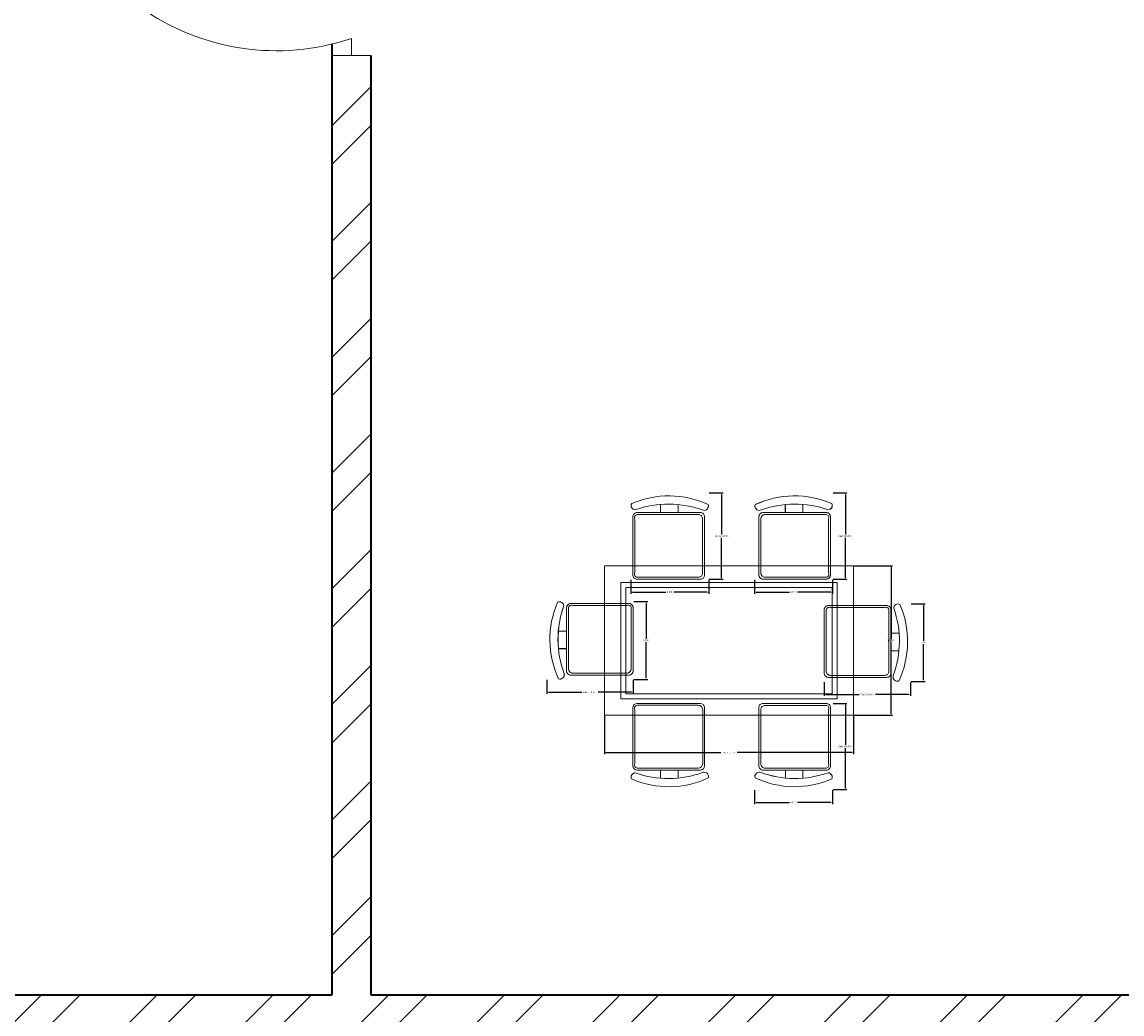
# Model space of a CAD drawing. Units: inches. Extents: x 2120 to 4013, y 1390 to 3019.
# Tile 31 of 59: x 2356 to 2484, y 2073 to 2188. Entities that reach past the tile are written whole.
import ezdxf

# ---------------------------------------------------------------- set-up
doc = ezdxf.new("R2010")
doc.units = ezdxf.units.IN
for name, color, linetype, lineweight in [('A-ANNO-DIMS', 2, 'Continuous', 18), ('A-DOOR', 3, 'Continuous', 18), ('A-FURN', 8, 'Continuous', 13), ('A-WALL', 7, 'Continuous', 35), ('A-WALL-PATT', 252, 'Continuous', 13)]:
    doc.layers.add(name, color=color, linetype=linetype, lineweight=lineweight)
doc.styles.get("Standard").update_dxf_attribs({"font": 'arial.ttf'})
doc.dimstyles.get("Standard").update_dxf_attribs({"dimtxt": 0.18, "dimasz": 0.18, "dimexe": 0.18, "dimexo": 0.0625, "dimgap": 0.09, "dimtad": 0, "dimtih": 1, "dimtoh": 1, "dimdec": 4, "dimzin": 0, "dimdsep": 46, "dimtxsty": 'Standard', "dimcen": 0.09, "dimadec": 0, "dimazin": 0, "dimtfac": 1, "dimtdec": 4, "dimtofl": 0, "dimtmove": 0, "dimatfit": 3, "dimfxl": 1, "dimtolj": 1, "dimtzin": 0, "dimarcsym": 0})

# ---------------------------------------------------------------- blocks, each defined once
blk = doc.blocks.new('DOOR-SWING-36IN-108p68DEG')
for p, q in [((38.25, 29.83), (33.75, 29.83)), ((33.75, 29.83), (36, 29.83)), ((36, 29.83), (36, 27.83)), ((36, 27.83), (0, 27.83)), ((36, 0), (36, 2)), ((33.75, 0), (38.25, 0)), ((38.25, 0), (36, 0))]:
    blk.add_line(p, q)
blk.add_arc((27.27, 27.83), 27.27, 180, 288.6764)
blk = doc.blocks.new('TABLE-DINING')
for points in [[(0, 17.41), (29.01, 17.41), (29.01, 0), (0, 0)], [(1.93, 15.47), (27.08, 15.47), (27.08, 1.93), (1.93, 1.93)], [(2.51, 14.89), (26.5, 14.89), (26.5, 2.51), (2.51, 2.51)]]:
    blk.add_lwpolyline(points, close=True)
blk = doc.blocks.new('CHAIR-DINING-01')
for points in [[(1.68, 0.62, -0.578392), (1.02, 0.02, -0.214524), (0.9, 8.94, -0.552014), (1.62, 8.52, 0.175809), (1.68, 0.62)], [(1.93, 8.29, -0.414214), (2.45, 8.81), (9.19, 8.81, -0.414214), (9.7, 8.29), (9.7, 0.96, -0.414214), (9.19, 0.45), (2.45, 0.45, -0.414214), (1.93, 0.96), (1.93, 8.29)], [(1.93, 3.54), (1.01, 3.54, 0.064759)]]:
    blk.add_lwpolyline(points, format="xyb")
blk.add_lwpolyline([(2.16, 8.29), (2.16, 1.19, 0.414214), (2.68, 0.68), (8.96, 0.68, 0.414214), (9.47, 1.19), (9.47, 8.29, 0.512069), (8.96, 8.58), (2.68, 8.58, 0.512069)], format="xyb", close=True)
blk.add_lwpolyline([(0.99, 5.59), (1.93, 5.59)])
blk = doc.blocks.new('CHAIR-DINING-02')
for points in [[(8.09, 8.52, -0.175809), (8.03, 0.62, 0.578392), (8.69, 0.02, 0.214524), (8.81, 8.94, 0.552014), (8.09, 8.52, -0.065079)], [(7.77, 8.29, 0.414214), (7.26, 8.81), (0.51, 8.81, 0.414214), (0, 8.29), (0, 0.96, 0.414214), (0.51, 0.45), (7.26, 0.45, 0.414214), (7.77, 0.96), (7.77, 8.29)], [(7.77, 3.54), (8.7, 3.54, -0.064759)]]:
    blk.add_lwpolyline(points, format="xyb")
blk.add_lwpolyline([(7.54, 8.29), (7.54, 1.19, -0.414214), (7.03, 0.68), (0.74, 0.68, -0.414214), (0.23, 1.19), (0.23, 8.29, -0.512069), (0.74, 8.58), (7.03, 8.58, -0.512069)], format="xyb", close=True)
blk.add_lwpolyline([(8.72, 5.59), (7.77, 5.59)])
blk = doc.blocks.new('CHAIR-DINING-03')
for points in [[(8.29, 1.93, 0.414214), (8.81, 2.45), (8.81, 9.19, 0.414214), (8.29, 9.7), (0.96, 9.7, 0.414214), (0.45, 9.19), (0.45, 2.45, 0.414214), (0.96, 1.93), (8.29, 1.93)], [(8.52, 1.62, -0.175809), (0.62, 1.68, 0.578392), (0.02, 1.02, 0.214524), (8.94, 0.9, 0.552014), (8.52, 1.62, -0.065079)], [(3.54, 1.93), (3.54, 1.01, -0.064759)]]:
    blk.add_lwpolyline(points, format="xyb")
blk.add_lwpolyline([(8.29, 2.16), (1.19, 2.16, -0.414214), (0.68, 2.68), (0.68, 8.96, -0.414214), (1.19, 9.47), (8.29, 9.47, -0.512069), (8.58, 8.96), (8.58, 2.68, -0.512069)], format="xyb", close=True)
blk.add_lwpolyline([(5.59, 0.99), (5.59, 1.93)])
blk = doc.blocks.new('CHAIR-DINING-09')
for points in [[(0.47, 8.09, -0.175809), (8.38, 8.03, 0.578392), (8.97, 8.69, 0.214524), (0.06, 8.81, 0.552014), (0.47, 8.09, -0.065079)], [(8.04, 7.77), (0.71, 7.77, 0.414214), (0.19, 7.26), (0.19, 0.51, 0.414214), (0.71, 0), (8.04, 0, 0.414214), (8.55, 0.51), (8.55, 7.26, 0.414214), (8.04, 7.77)], [(5.46, 7.77), (5.46, 8.7, -0.064759)]]:
    blk.add_lwpolyline(points, format="xyb")
blk.add_lwpolyline([(3.41, 8.72), (3.41, 7.77)])
blk.add_lwpolyline([(0.71, 7.54), (7.81, 7.54, -0.414214), (8.32, 7.03), (8.32, 0.74, -0.414214), (7.81, 0.23), (0.71, 0.23, -0.512069), (0.42, 0.74), (0.42, 7.03, -0.512069)], format="xyb", close=True)
blk = doc.blocks.new('CHAIR-DINING-10')
for points in [[(0.62, 8.03, -0.578392), (0.02, 8.69, -0.214524), (8.94, 8.81, -0.552014), (8.52, 8.09, 0.175809), (0.62, 8.03)], [(8.29, 7.77, -0.414214), (8.81, 7.26), (8.81, 0.51, -0.414214), (8.29, 0), (0.96, 0, -0.414214), (0.45, 0.51), (0.45, 7.26, -0.414214), (0.96, 7.77), (8.29, 7.77)], [(3.54, 7.77), (3.54, 8.7, 0.064759)]]:
    blk.add_lwpolyline(points, format="xyb")
blk.add_lwpolyline([(5.59, 8.72), (5.59, 7.77)])
blk.add_lwpolyline([(8.29, 7.54), (1.19, 7.54, 0.414214), (0.68, 7.03), (0.68, 0.74, 0.414214), (1.19, 0.23), (8.29, 0.23, 0.512069), (8.58, 0.74), (8.58, 7.03, 0.512069)], format="xyb", close=True)
blk = doc.blocks.new('CHAIR-DINING-11')
for points in [[(0.47, 8.09, -0.175809), (8.38, 8.03, 0.578392), (8.97, 8.69, 0.214524), (0.06, 8.81, 0.552014), (0.47, 8.09, -0.065079)], [(8.04, 7.77), (0.71, 7.77, 0.414214), (0.19, 7.26), (0.19, 0.51, 0.414214), (0.71, 0), (8.04, 0, 0.414214), (8.55, 0.51), (8.55, 7.26, 0.414214), (8.04, 7.77)], [(5.46, 7.77), (5.46, 8.7, -0.064759)]]:
    blk.add_lwpolyline(points, format="xyb")
blk.add_lwpolyline([(3.41, 8.72), (3.41, 7.77)])
blk.add_lwpolyline([(0.71, 7.54), (7.81, 7.54, -0.414214), (8.32, 7.03), (8.32, 0.74, -0.414214), (7.81, 0.23), (0.71, 0.23, -0.512069), (0.42, 0.74), (0.42, 7.03, -0.512069)], format="xyb", close=True)
blk = doc.blocks.new('CHAIR-DINING-12')
for points in [[(8.09, 8.52, -0.175809), (8.03, 0.62, 0.578392), (8.69, 0.02, 0.214524), (8.81, 8.94, 0.552014), (8.09, 8.52, -0.065079)], [(7.77, 8.29, 0.414214), (7.26, 8.81), (0.51, 8.81, 0.414214), (0, 8.29), (0, 0.96, 0.414214), (0.51, 0.45), (7.26, 0.45, 0.414214), (7.77, 0.96), (7.77, 8.29)], [(7.77, 3.54), (8.7, 3.54, -0.064759)]]:
    blk.add_lwpolyline(points, format="xyb")
blk.add_lwpolyline([(7.54, 8.29), (7.54, 1.19, -0.414214), (7.03, 0.68), (0.74, 0.68, -0.414214), (0.23, 1.19), (0.23, 8.29, -0.512069), (0.74, 8.58), (7.03, 8.58, -0.512069)], format="xyb", close=True)
blk.add_lwpolyline([(8.72, 5.59), (7.77, 5.59)])
blk = doc.blocks.new('*D75')
at = {"layer": 'A-ANNO-DIMS', "color": 0, "lineweight": -2, "transparency": 16777216}
for p, q in [((2423.42, 2107.5), (2423.42, 2103.03)), ((2452.43, 2107.5), (2452.43, 2103.03)), ((2423.6, 2103.21), (2436.97, 2103.21)), ((2452.25, 2103.21), (2438.89, 2103.21))]:
    blk.add_line(p, q, dxfattribs=at)
at = {"layer": 'A-ANNO-DIMS', "color": 0, "transparency": 16777216}
for points in [[(2423.6, 2103.24), (2423.6, 2103.18), (2423.42, 2103.21)], [(2452.25, 2103.24), (2452.25, 2103.18), (2452.43, 2103.21)]]:
    blk.add_solid(points, dxfattribs=at)
at = {"layer": 'Defpoints', "color": 0, "transparency": 16777216}
for p in [(2423.42, 2107.56), (2452.43, 2107.56), (2452.43, 2103.21)]:
    blk.add_point(p, dxfattribs=at)
at = {"layer": 'A-ANNO-DIMS', "color": 0, "transparency": 16777216, "insert": (2437.93, 2103.21), "char_height": 0.18, "attachment_point": 5}
blk.add_mtext('\\A1;TABLE 29 TYP.', dxfattribs=at)
blk = doc.blocks.new('*D76')
at = {"layer": 'A-ANNO-DIMS', "color": 0, "lineweight": -2, "transparency": 16777216}
for p, q in [((2452.5, 2124.97), (2456.97, 2124.97)), ((2456.79, 2124.79), (2456.79, 2116.45)), ((2456.79, 2107.74), (2456.79, 2116.09)), ((2452.5, 2107.56), (2456.97, 2107.56))]:
    blk.add_line(p, q, dxfattribs=at)
at = {"layer": 'A-ANNO-DIMS', "color": 0, "transparency": 16777216}
for points in [[(2456.76, 2124.79), (2456.82, 2124.79), (2456.79, 2124.97)], [(2456.76, 2107.74), (2456.82, 2107.74), (2456.79, 2107.56)]]:
    blk.add_solid(points, dxfattribs=at)
at = {"layer": 'Defpoints', "color": 0, "transparency": 16777216}
for p in [(2452.43, 2124.97), (2456.79, 2124.97), (2452.43, 2107.56)]:
    blk.add_point(p, dxfattribs=at)
at = {"layer": 'A-ANNO-DIMS', "color": 0, "transparency": 16777216, "insert": (2456.79, 2116.27), "char_height": 0.18, "attachment_point": 5}
blk.add_mtext('\\A1;17 TYP.', dxfattribs=at)
blk = doc.blocks.new('*D81')
at = {"layer": 'A-ANNO-DIMS', "color": 0, "lineweight": -2, "transparency": 16777216}
for p, q in [((2416.73, 2111.68), (2416.73, 2110.06)), ((2426.77, 2111.68), (2426.77, 2110.06)), ((2416.91, 2110.24), (2420.8, 2110.24)), ((2426.59, 2110.24), (2422.7, 2110.24))]:
    blk.add_line(p, q, dxfattribs=at)
at = {"layer": 'A-ANNO-DIMS', "color": 0, "transparency": 16777216}
for points in [[(2416.91, 2110.27), (2416.91, 2110.21), (2416.73, 2110.24)], [(2426.59, 2110.27), (2426.59, 2110.21), (2426.77, 2110.24)]]:
    blk.add_solid(points, dxfattribs=at)
at = {"layer": 'Defpoints', "color": 0, "transparency": 16777216}
for p in [(2416.73, 2111.74), (2426.77, 2111.74), (2426.77, 2110.24)]:
    blk.add_point(p, dxfattribs=at)
at = {"layer": 'A-ANNO-DIMS', "color": 0, "transparency": 16777216, "insert": (2421.75, 2110.24), "char_height": 0.18, "attachment_point": 5}
blk.add_mtext('\\A1;CHAIR 10 TYP.', dxfattribs=at)
blk = doc.blocks.new('*D82')
at = {"layer": 'A-ANNO-DIMS', "color": 0, "lineweight": -2, "transparency": 16777216}
for p, q in [((2426.84, 2120.8), (2428.46, 2120.8)), ((2428.28, 2120.62), (2428.28, 2116.45)), ((2428.28, 2111.92), (2428.28, 2116.09)), ((2426.84, 2111.74), (2428.46, 2111.74))]:
    blk.add_line(p, q, dxfattribs=at)
at = {"layer": 'A-ANNO-DIMS', "color": 0, "transparency": 16777216}
for points in [[(2428.25, 2120.62), (2428.31, 2120.62), (2428.28, 2120.8)], [(2428.25, 2111.92), (2428.31, 2111.92), (2428.28, 2111.74)]]:
    blk.add_solid(points, dxfattribs=at)
at = {"layer": 'Defpoints', "color": 0, "transparency": 16777216}
for p in [(2426.77, 2120.8), (2428.28, 2120.8), (2426.77, 2111.74)]:
    blk.add_point(p, dxfattribs=at)
at = {"layer": 'A-ANNO-DIMS', "color": 0, "transparency": 16777216, "insert": (2428.28, 2116.27), "char_height": 0.18, "attachment_point": 5}
blk.add_mtext('\\A1;9 TYP.', dxfattribs=at)
blk = doc.blocks.new('*D85')
at = {"layer": 'A-ANNO-DIMS', "color": 0, "lineweight": -2, "transparency": 16777216}
for p, q in [((2450.03, 2108.95), (2451.65, 2108.95)), ((2451.47, 2108.77), (2451.47, 2104.11)), ((2451.47, 2099.09), (2451.47, 2103.75)), ((2450.03, 2098.91), (2451.65, 2098.91))]:
    blk.add_line(p, q, dxfattribs=at)
at = {"layer": 'A-ANNO-DIMS', "color": 0, "transparency": 16777216}
for points in [[(2451.44, 2108.77), (2451.5, 2108.77), (2451.47, 2108.95)], [(2451.44, 2099.09), (2451.5, 2099.09), (2451.47, 2098.91)]]:
    blk.add_solid(points, dxfattribs=at)
at = {"layer": 'Defpoints', "color": 0, "transparency": 16777216}
for p in [(2449.96, 2108.95), (2451.47, 2108.95), (2449.96, 2098.91)]:
    blk.add_point(p, dxfattribs=at)
at = {"layer": 'A-ANNO-DIMS', "color": 0, "transparency": 16777216, "insert": (2451.47, 2103.93), "char_height": 0.18, "attachment_point": 5}
blk.add_mtext('\\A1;CHAIR 10 TYP.', dxfattribs=at)
blk = doc.blocks.new('*D86')
at = {"layer": 'A-ANNO-DIMS', "color": 0, "lineweight": -2, "transparency": 16777216}
for p, q in [((2440.91, 2098.85), (2440.91, 2097.22)), ((2449.96, 2098.85), (2449.96, 2097.22)), ((2441.09, 2097.4), (2444.98, 2097.4)), ((2449.78, 2097.4), (2445.9, 2097.4))]:
    blk.add_line(p, q, dxfattribs=at)
at = {"layer": 'A-ANNO-DIMS', "color": 0, "transparency": 16777216}
for points in [[(2441.09, 2097.43), (2441.09, 2097.37), (2440.91, 2097.4)], [(2449.78, 2097.43), (2449.78, 2097.37), (2449.96, 2097.4)]]:
    blk.add_solid(points, dxfattribs=at)
at = {"layer": 'Defpoints', "color": 0, "transparency": 16777216}
for p in [(2440.91, 2098.91), (2449.96, 2098.91), (2449.96, 2097.4)]:
    blk.add_point(p, dxfattribs=at)
at = {"layer": 'A-ANNO-DIMS', "color": 0, "transparency": 16777216, "insert": (2445.44, 2097.4), "char_height": 0.18, "attachment_point": 5}
blk.add_mtext('\\A1;9 TYP.', dxfattribs=at)
blk = doc.blocks.new('*D97')
at = {"layer": 'A-ANNO-DIMS', "color": 0, "lineweight": -2, "transparency": 16777216}
for p, q in [((2435.63, 2133.44), (2437.25, 2133.44)), ((2437.07, 2133.26), (2437.07, 2128.6)), ((2437.07, 2123.57), (2437.07, 2128.23)), ((2435.63, 2123.39), (2437.25, 2123.39))]:
    blk.add_line(p, q, dxfattribs=at)
at = {"layer": 'A-ANNO-DIMS', "color": 0, "transparency": 16777216}
for points in [[(2437.04, 2133.26), (2437.1, 2133.26), (2437.07, 2133.44)], [(2437.04, 2123.57), (2437.1, 2123.57), (2437.07, 2123.39)]]:
    blk.add_solid(points, dxfattribs=at)
at = {"layer": 'Defpoints', "color": 0, "transparency": 16777216}
for p in [(2435.57, 2133.44), (2437.07, 2133.44), (2435.57, 2123.39)]:
    blk.add_point(p, dxfattribs=at)
at = {"layer": 'A-ANNO-DIMS', "color": 0, "transparency": 16777216, "insert": (2437.07, 2128.41), "char_height": 0.18, "attachment_point": 5}
blk.add_mtext('\\A1;CHAIR 10 TYP.', dxfattribs=at)
blk = doc.blocks.new('*D98')
at = {"layer": 'A-ANNO-DIMS', "color": 0, "lineweight": -2, "transparency": 16777216}
for p, q in [((2426.51, 2123.33), (2426.51, 2121.71)), ((2435.57, 2123.33), (2435.57, 2121.71)), ((2426.69, 2121.89), (2430.58, 2121.89)), ((2435.39, 2121.89), (2431.5, 2121.89))]:
    blk.add_line(p, q, dxfattribs=at)
at = {"layer": 'A-ANNO-DIMS', "color": 0, "transparency": 16777216}
for points in [[(2426.69, 2121.92), (2426.69, 2121.86), (2426.51, 2121.89)], [(2435.39, 2121.92), (2435.39, 2121.86), (2435.57, 2121.89)]]:
    blk.add_solid(points, dxfattribs=at)
at = {"layer": 'Defpoints', "color": 0, "transparency": 16777216}
for p in [(2426.51, 2123.39), (2435.57, 2123.39), (2435.57, 2121.89)]:
    blk.add_point(p, dxfattribs=at)
at = {"layer": 'A-ANNO-DIMS', "color": 0, "transparency": 16777216, "insert": (2431.04, 2121.89), "char_height": 0.18, "attachment_point": 5}
blk.add_mtext('\\A1;9 TYP.', dxfattribs=at)
blk = doc.blocks.new('*D99')
at = {"layer": 'A-ANNO-DIMS', "color": 0, "lineweight": -2, "transparency": 16777216}
for p, q in [((2450.03, 2133.44), (2451.65, 2133.44)), ((2451.47, 2133.26), (2451.47, 2128.6)), ((2451.47, 2123.57), (2451.47, 2128.23)), ((2450.03, 2123.39), (2451.65, 2123.39))]:
    blk.add_line(p, q, dxfattribs=at)
at = {"layer": 'A-ANNO-DIMS', "color": 0, "transparency": 16777216}
for points in [[(2451.44, 2133.26), (2451.5, 2133.26), (2451.47, 2133.44)], [(2451.44, 2123.57), (2451.5, 2123.57), (2451.47, 2123.39)]]:
    blk.add_solid(points, dxfattribs=at)
at = {"layer": 'Defpoints', "color": 0, "transparency": 16777216}
for p in [(2449.96, 2133.44), (2451.47, 2133.44), (2449.96, 2123.39)]:
    blk.add_point(p, dxfattribs=at)
at = {"layer": 'A-ANNO-DIMS', "color": 0, "transparency": 16777216, "insert": (2451.47, 2128.41), "char_height": 0.18, "attachment_point": 5}
blk.add_mtext('\\A1;CHAIR 10 TYP.', dxfattribs=at)
blk = doc.blocks.new('*D100')
at = {"layer": 'A-ANNO-DIMS', "color": 0, "lineweight": -2, "transparency": 16777216}
for p, q in [((2440.91, 2123.33), (2440.91, 2121.71)), ((2449.96, 2123.33), (2449.96, 2121.71)), ((2441.09, 2121.89), (2444.98, 2121.89)), ((2449.78, 2121.89), (2445.9, 2121.89))]:
    blk.add_line(p, q, dxfattribs=at)
at = {"layer": 'A-ANNO-DIMS', "color": 0, "transparency": 16777216}
for points in [[(2441.09, 2121.92), (2441.09, 2121.86), (2440.91, 2121.89)], [(2449.78, 2121.92), (2449.78, 2121.86), (2449.96, 2121.89)]]:
    blk.add_solid(points, dxfattribs=at)
at = {"layer": 'Defpoints', "color": 0, "transparency": 16777216}
for p in [(2440.91, 2123.39), (2449.96, 2123.39), (2449.96, 2121.89)]:
    blk.add_point(p, dxfattribs=at)
at = {"layer": 'A-ANNO-DIMS', "color": 0, "transparency": 16777216, "insert": (2445.44, 2121.89), "char_height": 0.18, "attachment_point": 5}
blk.add_mtext('\\A1;9 TYP.', dxfattribs=at)
blk = doc.blocks.new('*D103')
at = {"layer": 'A-ANNO-DIMS', "color": 0, "lineweight": -2, "transparency": 16777216}
for p, q in [((2449.01, 2111.43), (2449.01, 2109.81)), ((2459.05, 2111.43), (2459.05, 2109.81)), ((2449.19, 2109.99), (2453.08, 2109.99)), ((2458.87, 2109.99), (2454.98, 2109.99))]:
    blk.add_line(p, q, dxfattribs=at)
at = {"layer": 'A-ANNO-DIMS', "color": 0, "transparency": 16777216}
for points in [[(2449.19, 2110.02), (2449.19, 2109.96), (2449.01, 2109.99)], [(2458.87, 2110.02), (2458.87, 2109.96), (2459.05, 2109.99)]]:
    blk.add_solid(points, dxfattribs=at)
at = {"layer": 'Defpoints', "color": 0, "transparency": 16777216}
for p in [(2449.01, 2111.49), (2459.05, 2111.49), (2459.05, 2109.99)]:
    blk.add_point(p, dxfattribs=at)
at = {"layer": 'A-ANNO-DIMS', "color": 0, "transparency": 16777216, "insert": (2454.03, 2109.99), "char_height": 0.18, "attachment_point": 5}
blk.add_mtext('\\A1;CHAIR 10 TYP.', dxfattribs=at)
blk = doc.blocks.new('*D104')
at = {"layer": 'A-ANNO-DIMS', "color": 0, "lineweight": -2, "transparency": 16777216}
for p, q in [((2459.11, 2120.55), (2460.74, 2120.55)), ((2460.56, 2120.37), (2460.56, 2116.2)), ((2460.56, 2111.67), (2460.56, 2115.84)), ((2459.11, 2111.49), (2460.74, 2111.49))]:
    blk.add_line(p, q, dxfattribs=at)
at = {"layer": 'A-ANNO-DIMS', "color": 0, "transparency": 16777216}
for points in [[(2460.53, 2120.37), (2460.59, 2120.37), (2460.56, 2120.55)], [(2460.53, 2111.67), (2460.59, 2111.67), (2460.56, 2111.49)]]:
    blk.add_solid(points, dxfattribs=at)
at = {"layer": 'Defpoints', "color": 0, "transparency": 16777216}
for p in [(2459.05, 2120.55), (2460.56, 2120.55), (2459.05, 2111.49)]:
    blk.add_point(p, dxfattribs=at)
at = {"layer": 'A-ANNO-DIMS', "color": 0, "transparency": 16777216, "insert": (2460.56, 2116.02), "char_height": 0.18, "attachment_point": 5}
blk.add_mtext('\\A1;9 TYP.', dxfattribs=at)

msp = doc.modelspace()

# ---------------------------------------------------------------- hatches: boundary and pattern name
at = {"layer": 'A-WALL-PATT'}
h = msp.add_hatch(dxfattribs=at)
h.set_pattern_fill('ANSI32', color=256)
h.paths.add_polyline_path([(2271.7331, 2122.6377), (2262.7331, 2122.6377), (2262.7331, 2040.3893), (2267.2331, 2040.3893), (2271.7331, 2040.3893), (2271.7331, 2044.8856), (2271.7331, 2070.531), (2391.7331, 2070.531), (2391.7331, 1926.5306), (2388.3993, 1926.5306), (2388.3993, 1922.531), (2395.7331, 1922.531), (2395.7331, 1992.531), (2400.4511, 1992.531), (2400.4511, 1997.0306), (2395.7331, 1997.0306), (2395.7331, 2070.531), (2443.7331, 2070.531), (2443.7331, 2046.1368), (2448.2331, 2046.1368), (2448.2331, 2070.531), (2580.2331, 2070.531), (2580.2331, 1997.0306), (2492.9076, 1997.0306), (2492.9076, 1992.531), (2580.2331, 1992.531), (2580.2331, 1983.9368), (2589.2331, 1983.9368), (2589.2331, 2070.531), (2589.2331, 2075.0306), (2396.2331, 2075.0306), (2396.2331, 2184.3565), (2393.9831, 2184.3565), (2391.7331, 2184.3565), (2391.7331, 2075.0306), (2271.7331, 2075.0306)])
h.paths.add_polyline_path([(2724.7331, 2138.0306), (2628.7331, 2138.0306), (2628.7331, 2070.5306), (2628.7331, 2067.0987), (2633.2331, 2067.0987), (2637.7331, 2067.0987), (2637.7331, 2070.531), (2657.3413, 2070.531), (2657.3413, 2079.5306), (2637.7331, 2079.5306), (2637.7331, 2129.031), (2715.7331, 2129.031), (2715.7331, 2079.5306), (2698.0378, 2079.5306), (2698.0378, 2070.531), (2715.7331, 2070.531), (2715.7331, 2012.1531), (2720.2331, 2012.1531), (2724.7331, 2012.1531)])
h.paths.add_polyline_path([(2724.7331, 2213.031), (2831.3209, 2213.031), (2831.3209, 2215.281), (2831.3209, 2217.5306), (2724.7331, 2217.5306), (2724.7331, 2343.531), (2751.8755, 2343.531), (2751.8755, 2352.5306), (2715.7331, 2352.5306), (2715.7331, 2138.031), (2724.7331, 2138.031)])
h.paths.add_polyline_path([(2902.53, 2352.5306), (2811.8755, 2352.5306), (2811.8755, 2343.531), (2867.2331, 2343.531), (2867.2331, 2217.5306), (2863.6364, 2217.5306), (2863.6364, 2213.031), (2871.7331, 2213.031), (2871.7331, 2217.531), (2871.7331, 2343.531), (2902.53, 2343.531)])
h.paths.add_polyline_path([(3009.7331, 2352.5306), (2938.53, 2352.5306), (2938.53, 2343.531), (2966.2331, 2343.531), (2966.2331, 2242.3281), (2968.4831, 2242.3281), (2970.7331, 2242.3281), (2970.7331, 2343.531), (3009.7331, 2343.531)])
h.paths.add_polyline_path([(3009.7331, 2217.5306), (2970.7331, 2217.5306), (2970.7331, 2220.5422), (2968.4831, 2220.5422), (2966.2331, 2220.5422), (2966.2331, 2217.5306), (2911.7752, 2217.5306), (2907.7331, 2217.5306), (2907.7331, 2213.0306), (2907.7331, 2194.9663), (2912.2331, 2194.9663), (2912.2331, 2213.031), (2970.7331, 2213.031), (3000.7331, 2213.031), (3000.7331, 2205.523), (3009.7331, 2205.523)])
h.paths.add_polyline_path([(3009.7331, 2181.5227), (3000.7331, 2181.5227), (3000.7331, 2165.0306), (2912.2331, 2165.0306), (2912.2331, 2170.8202), (2907.7331, 2170.8202), (2907.7331, 2165.0306), (2899.5169, 2165.0306), (2899.5169, 2162.7806), (2899.5169, 2160.531), (2907.7331, 2160.531), (2907.7331, 2137.3432), (2912.2331, 2137.3432), (2912.2331, 2160.531), (3000.7331, 2160.531), (3000.7331, 2150.4993), (3009.7331, 2150.4993)])
h.paths.add_polyline_path([(3009.7331, 2126.499), (3005.2331, 2126.499), (3000.7331, 2126.499), (3000.7331, 2112.5306), (2912.2331, 2112.5306), (2912.2331, 2115.6036), (2907.7331, 2115.6036), (2907.7331, 2108.031), (3000.7331, 2108.031), (3000.7331, 2084.7256), (3009.7331, 2084.7256)], flags=17)
h.paths.add_polyline_path([(3009.7331, 1971.531), (3009.7331, 2024.7253), (3000.7331, 2024.7253), (3000.7331, 2006.4153), (3000.7331, 1971.5306), (2864.2331, 1971.5306), (2864.2331, 2160.531), (2868.0522, 2160.531), (2868.0522, 2165.0306), (2859.7331, 2165.0306), (2859.7331, 1971.5306), (2724.7331, 1971.5306), (2724.7331, 1977.7012), (2715.7331, 1977.7012), (2715.7331, 1962.5306), (2715.7331, 1950.9035), (2720.2331, 1950.9035), (2724.7331, 1950.9035), (2724.7331, 1962.531), (2855.2331, 1962.531), (2859.7331, 1962.531), (2859.7331, 1835.031), (2864.2331, 1834.8158), (2864.2331, 1962.531), (2958.7331, 1962.531), (2958.7331, 1937.0925), (2963.2331, 1937.0925), (2963.2331, 1962.531), (3000.7331, 1962.531), (3009.7331, 1962.531)])
h.paths.add_polyline_path([(2724.7331, 1728.531), (2822.7164, 1728.531), (2822.7164, 1733.0306), (2724.7331, 1733.0306), (2724.7331, 1779.3416), (2715.7331, 1779.3416), (2715.7331, 1581.531), (2753.02, 1581.531), (2753.02, 1586.031), (2753.02, 1590.5306), (2724.7331, 1590.5306)])
h.paths.add_polyline_path([(2864.2331, 1590.531), (2864.2331, 1787.031), (2868.4075, 1787.031), (2868.4075, 1791.5306), (2859.7331, 1791.5306), (2859.7331, 1739.0306), (2859.7331, 1733.0306), (2854.3125, 1733.0306), (2854.3125, 1728.531), (2859.7331, 1728.531), (2859.7331, 1590.5306), (2813.02, 1590.5306), (2813.02, 1581.531), (2868.4123, 1581.531), (2868.4123, 1583.781), (2868.4123, 1586.0306), (2864.2331, 1586.0306)])
h.paths.add_polyline_path([(3009.7331, 1754.6619), (3000.7331, 1754.6619), (3000.7331, 1739.0306), (2912.2331, 1739.0306), (2912.2331, 1742.2257), (2907.7331, 1742.2257), (2907.7331, 1739.0306), (2907.7331, 1734.531), (3000.7331, 1734.531), (3000.7331, 1590.5306), (3000.7331, 1586.0306), (2971.3921, 1586.0306), (2971.3921, 1581.531), (3009.7331, 1581.531)])
h.paths.add_polyline_path([(2911.3921, 1583.781), (2911.3921, 1586.0306), (2891.2138, 1586.0306), (2891.2138, 1581.531), (2911.3921, 1581.531)])
h.paths.add_polyline_path([(3009.7331, 1799.8422), (3000.7331, 1799.8422), (3000.7331, 1791.5306), (2912.2331, 1791.5306), (2912.2331, 1796.3264), (2909.9831, 1796.3264), (2907.7331, 1796.3264), (2907.7331, 1791.5306), (2902.7033, 1791.5306), (2902.7033, 1787.031), (2907.7331, 1787.031), (2907.7331, 1761.1622), (2912.2331, 1761.1622), (2912.2331, 1787.031), (3000.7331, 1787.031), (3000.7331, 1778.6622), (3009.7331, 1778.6622)])
h.paths.add_polyline_path([(3009.7331, 1839.5306), (2963.2331, 1839.5306), (2963.2331, 1842.8629), (2960.9831, 1842.8629), (2958.7331, 1842.8629), (2958.7331, 1839.5306), (2907.7331, 1839.5306), (2907.7331, 1814.4599), (2912.2331, 1814.4599), (2912.2331, 1835.031), (3000.7331, 1835.031), (3000.7331, 1823.8425), (3009.7331, 1823.8425), (3009.7331, 1835.031)])
h.paths.add_polyline_path([(2963.2331, 1901.0922), (2960.9831, 1901.0922), (2958.7331, 1901.0922), (2958.7331, 1862.8843), (2963.2331, 1862.8843)], flags=17)
h.paths.add_polyline_path([(2724.7331, 1891.9826), (2724.7331, 1914.3416), (2715.7331, 1914.3416), (2715.7331, 1783.8416), (2637.7331, 1783.8416), (2637.7331, 1914.3416), (2628.7331, 1914.3416), (2624.7701, 1914.3416), (2624.7701, 1909.8416), (2624.7701, 1905.3419), (2628.7331, 1905.3419), (2628.7331, 1876.9915), (2628.7331, 1779.3419), (2637.7331, 1779.3419), (2715.7331, 1779.3419), (2724.7331, 1779.3419), (2724.7331, 1835.031)])
h.paths.add_polyline_path([(2637.7331, 1731.531), (2637.7331, 1779.3416), (2628.7331, 1779.3416), (2628.7331, 1731.5306), (2589.2331, 1731.5306), (2535.9814, 1731.5306), (2496.7331, 1731.5306), (2496.7331, 1725.6876), (2498.9831, 1725.6876), (2501.2331, 1725.6876), (2501.2331, 1727.031), (2628.7331, 1727.031), (2628.7331, 1680.4203), (2628.7331, 1590.5306), (2628.7331, 1586.0306), (2604.1361, 1586.0306), (2604.1361, 1581.531), (2637.7331, 1581.531), (2637.7331, 1590.531)])

# ---------------------------------------------------------------- linework, layer by layer
at = {"layer": 'A-FURN'}
for points in [[(2441.5657, 2131.4213, -0.57839206), (2440.9671, 2132.0795, -0.21452438), (2449.8864, 2132.1992, -0.55201397), (2449.4674, 2131.4811, 0.1758092), (2441.5657, 2131.4213)], [(2444.4776, 2131.164), (2444.4776, 2132.0917, 0.06475861)], [(2449.2366, 2131.164, -0.41421356), (2449.7498, 2130.6508), (2449.7498, 2123.9058, -0.41421356), (2449.2366, 2123.3926), (2441.9009, 2123.3926, -0.41421356), (2441.3877, 2123.9058), (2441.3877, 2130.6508, -0.41421356), (2441.9009, 2131.164), (2449.2366, 2131.164)], [(2418.745, 2112.4, -0.57839206), (2418.0868, 2111.8014, -0.21452438), (2417.9671, 2120.7208, -0.55201397), (2418.6852, 2120.3017, 0.17580937), (2418.745, 2112.4)], [(2419.0023, 2120.0709, -0.41421356), (2419.5156, 2120.5841), (2426.2606, 2120.5841, -0.41421356), (2426.7738, 2120.0709), (2426.7738, 2112.7353, -0.41421356), (2426.2606, 2112.222), (2419.5156, 2112.222, -0.41421356), (2419.0023, 2112.7353), (2419.0023, 2120.0709)], [(2419.0023, 2115.3119), (2418.0746, 2115.3119, 0.06475861)], [(2434.5782, 2101.1811), (2427.2425, 2101.1811, -0.41421356), (2426.7293, 2101.6943), (2426.7293, 2108.4393, -0.41421356), (2427.2425, 2108.9525), (2434.5782, 2108.9525, -0.41421356), (2435.0914, 2108.4393), (2435.0914, 2101.6943, -0.41421356), (2434.5782, 2101.1811)], [(2434.5782, 2101.1808), (2427.2426, 2101.1808, -0.41421356), (2426.7293, 2101.694), (2426.7293, 2108.439, -0.41421356), (2427.2426, 2108.9522), (2434.5782, 2108.9522, -0.41421356), (2435.0914, 2108.439), (2435.0914, 2101.694, -0.41421356), (2434.5782, 2101.1808)], [(2432.0016, 2101.1811), (2432.0016, 2100.2533, 0.06475861)], [(2432.0016, 2101.1808), (2432.0016, 2100.253, 0.06475861)], [(2434.9134, 2100.9238, -0.57839206), (2435.5121, 2100.2656, -0.21452438), (2426.5927, 2100.1459, -0.55201397), (2427.0117, 2100.8639, 0.17580929), (2434.9134, 2100.9238)], [(2434.9135, 2100.9235, -0.57839206), (2435.5121, 2100.2652, -0.21452438), (2426.5927, 2100.1456, -0.55201397), (2427.0118, 2100.8636, 0.17580929), (2434.9135, 2100.9235)]]:
    msp.add_lwpolyline(points, format="xyb", dxfattribs=at)
for points in [[(2446.5309, 2132.1086), (2446.5309, 2131.164)], [(2418.0578, 2117.3653), (2419.0023, 2117.3653)], [(2429.9482, 2100.2365), (2429.9482, 2101.1811)], [(2429.9482, 2100.2362), (2429.9482, 2101.1808)]]:
    msp.add_lwpolyline(points, dxfattribs=at)
for points in [[(2449.2335, 2130.9328), (2442.1321, 2130.9328, 0.41421356), (2441.6189, 2130.4196), (2441.6189, 2124.137, 0.41421356), (2442.1321, 2123.6238), (2449.2335, 2123.6238, 0.51206948), (2449.5186, 2124.137), (2449.5186, 2130.4196, 0.51206948)], [(2419.2336, 2120.0678), (2419.2336, 2112.9665, 0.41421356), (2419.7468, 2112.4533), (2426.0294, 2112.4533, 0.41421356), (2426.5426, 2112.9665), (2426.5426, 2120.0678, 0.51206948), (2426.0294, 2120.3529), (2419.7468, 2120.3529, 0.51206948)], [(2427.2457, 2101.4123), (2434.347, 2101.4123, 0.41421356), (2434.8602, 2101.9255), (2434.8602, 2108.2081, 0.41421356), (2434.347, 2108.7213), (2427.2457, 2108.7213, 0.51206948), (2426.9605, 2108.2081), (2426.9605, 2101.9255, 0.51206948)], [(2427.2457, 2101.412), (2434.347, 2101.412, 0.41421356), (2434.8602, 2101.9252), (2434.8602, 2108.2078, 0.41421356), (2434.347, 2108.721), (2427.2457, 2108.721, 0.51206948), (2426.9606, 2108.2078), (2426.9606, 2101.9252, 0.51206948)]]:
    msp.add_lwpolyline(points, format="xyb", close=True, dxfattribs=at)
at = {"layer": 'A-WALL'}
for p, q in [((2391.7331, 2075.031), (2391.7331, 2185.7025)), ((2391.7331, 2075.0306), (2391.7331, 2185.7022)), ((2396.2331, 2184.3568), (2396.2331, 2075.031)), ((2396.2331, 2184.3565), (2396.2331, 2075.0306)), ((2271.7331, 2075.031), (2391.7331, 2075.031)), ((2271.7331, 2075.031), (2391.7331, 2075.031)), ((2271.7331, 2075.0306), (2391.7331, 2075.0306)), ((2271.7331, 2075.0306), (2391.7331, 2075.0306)), ((2396.2331, 2075.031), (2589.2331, 2075.031)), ((2396.2331, 2075.0306), (2589.2331, 2075.0306))]:
    msp.add_line(p, q, dxfattribs=at)

# ---------------------------------------------------------------- block references
at = {"layer": 'A-DOOR'}
for p in [(2357.9831, 2184.3568), (2357.9831, 2184.3565)]:
    msp.add_blockref('DOOR-SWING-36IN-108p68DEG', p, dxfattribs=at)
at = {"layer": 'A-FURN'}
for name, p in [('CHAIR-DINING-09', (2426.5371, 2123.3929)), ('CHAIR-DINING-11', (2426.5371, 2123.3926)), ('CHAIR-DINING-10', (2440.9425, 2123.3929)), ('TABLE-DINING', (2423.4234, 2107.5627)), ('TABLE-DINING', (2423.4234, 2107.5624)), ('CHAIR-DINING-01', (2417.0693, 2111.7765)), ('CHAIR-DINING-02', (2449.0062, 2111.5256)), ('CHAIR-DINING-12', (2449.0062, 2111.5253)), ('CHAIR-DINING-03', (2440.9425, 2099.248)), ('CHAIR-DINING-03', (2440.9425, 2099.2477))]:
    msp.add_blockref(name, p, dxfattribs=at)

# ---------------------------------------------------------------- dimensions: what is measured, and where the dimension line sits
at = {"layer": 'A-ANNO-DIMS'}
for base, p1, p2, text, picture, middle in [((2437.0748, 2133.4371), (2435.5682, 2123.3929), (2435.5682, 2133.4371), 'CHAIR <> TYP.', '*D97', (2437.0748, 2128.415)), ((2451.471, 2133.4371), (2449.9644, 2123.3929), (2449.9644, 2133.4371), 'CHAIR <> TYP.', '*D99', (2451.471, 2128.415)), ((2456.7858, 2124.9691), (2452.4342, 2107.5627), (2452.4342, 2124.9691), '<> TYP.', '*D76', (2456.7858, 2116.2659)), ((2428.2804, 2120.7985), (2426.7738, 2111.7449), (2426.7738, 2120.7985), '<> TYP.', '*D82', (2428.2804, 2116.2717)), ((2460.557, 2120.5472), (2459.0504, 2111.4937), (2459.0504, 2120.5472), '<> TYP.', '*D104', (2460.557, 2116.0205)), ((2451.471, 2108.9525), (2449.9644, 2098.9083), (2449.9644, 2108.9525), 'CHAIR <> TYP.', '*D85', (2451.471, 2103.9304))]:
    dim = msp.add_linear_dim(base=base, p1=p1, p2=p2, angle=90, text=text, dimstyle='Standard', override={"dimdec": 0, "dimlfac": 1, "dimrnd": 0, "dimzin": 0, "dimdsep": 46, "dimlunit": 2}, dxfattribs=at)
    dim.commit()
    dim.dimension.update_dxf_attribs({"geometry": picture, "text_midpoint": middle})
for base, p1, p2, text, picture, middle in [((2435.5682, 2121.8862), (2426.5147, 2123.3929), (2435.5682, 2123.3929), '<> TYP.', '*D98', (2431.0415, 2121.8862)), ((2449.9644, 2121.8862), (2440.9109, 2123.3929), (2449.9644, 2123.3929), '<> TYP.', '*D100', (2445.4377, 2121.8862)), ((2426.7738, 2110.2383), (2416.7296, 2111.7449), (2426.7738, 2111.7449), 'CHAIR <> TYP.', '*D81', (2421.7517, 2110.2383)), ((2459.0504, 2109.9871), (2449.0062, 2111.4937), (2459.0504, 2111.4937), 'CHAIR <> TYP.', '*D103', (2454.0283, 2109.9871)), ((2452.4342, 2103.2111), (2423.4234, 2107.5627), (2452.4342, 2107.5627), 'TABLE <> TYP.', '*D75', (2437.9288, 2103.2111)), ((2449.9644, 2097.4017), (2440.9109, 2098.9083), (2449.9644, 2098.9083), '<> TYP.', '*D86', (2445.4377, 2097.4017))]:
    dim = msp.add_linear_dim(base=base, p1=p1, p2=p2, text=text, dimstyle='Standard', override={"dimdec": 0, "dimlfac": 1, "dimrnd": 0, "dimzin": 0, "dimdsep": 46, "dimlunit": 2}, dxfattribs=at)
    dim.commit()
    dim.dimension.update_dxf_attribs({"geometry": picture, "text_midpoint": middle})

doc.saveas('drawing.dxf')
